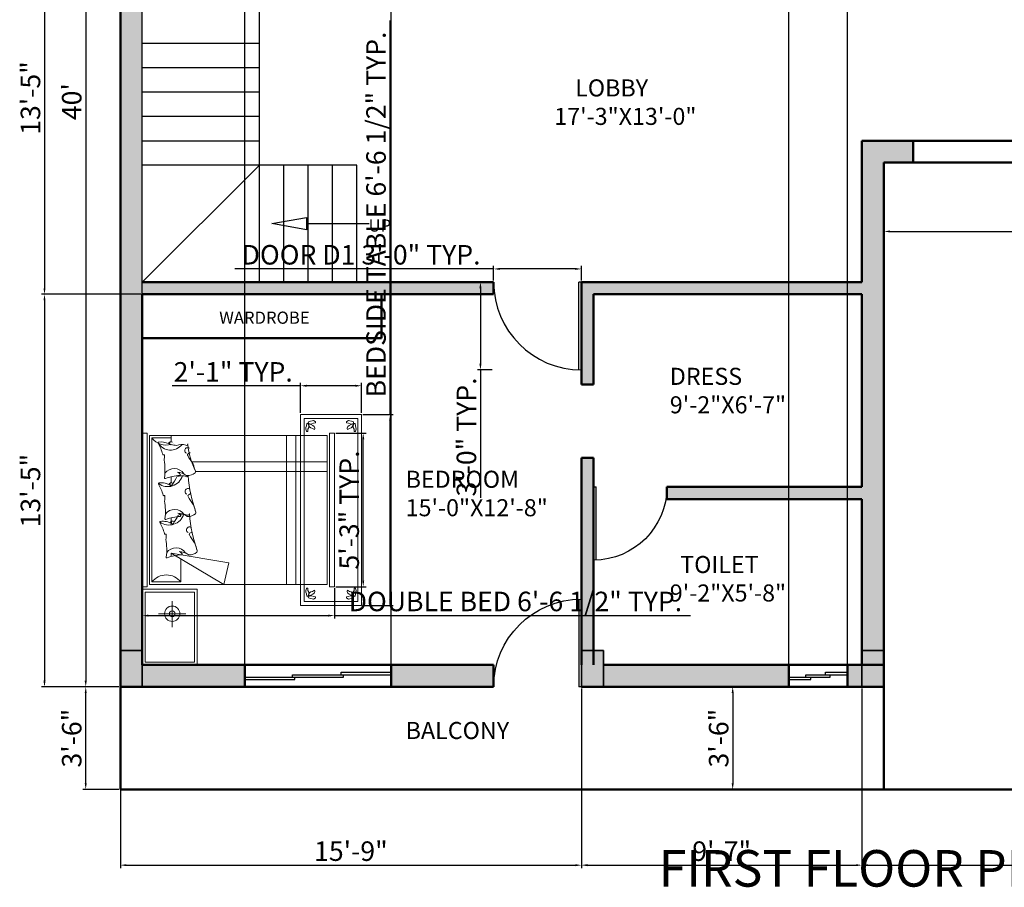
# Model space of a CAD drawing. Units: inches. Extents: x 1770 to 3141, y 984 to 1614.
# Tile 10 of 12: x 2468 to 2871, y 1003 to 1359. Entities that reach past the tile are written whole.
import ezdxf

# ---------------------------------------------------------------- set-up
doc = ezdxf.new("R2010")
doc.units = ezdxf.units.IN
for name, color, linetype, lineweight in [('A-ANNO-DIMS', 2, 'Continuous', 18), ('A-ANNO-TEXT', 7, 'Continuous', 18), ('A-AREA-IDEN', 3, 'Continuous', 18), ('A-COLS', 1, 'Continuous', 35), ('A-DOOR', 4, 'Continuous', 25), ('A-FLOR-STRS', 7, 'Continuous', 25), ('A-FURN', 8, 'Continuous', 18), ('A-GLAZ', 5, 'Continuous', 25), ('A-WALL', 7, 'Continuous', 50), ('A-WALL-PATT', 8, 'Continuous', 13)]:
    doc.layers.add(name, color=color, linetype=linetype, lineweight=lineweight)
doc.styles.get("Standard").update_dxf_attribs({"font": 'arial.ttf'})
doc.dimstyles.new('ISO-25', dxfattribs={"dimtxt": 8, "dimasz": 2.5, "dimexe": 1.25, "dimexo": 0.625, "dimtad": 1, "dimdec": 1, "dimlunit": 3, "dimtxsty": 'Standard', "dimcen": 2.5, "dimclrt": 1, "dimadec": 0, "dimazin": 0, "dimtfac": 1, "dimtdec": 1, "dimtmove": 0, "dimatfit": 3, "dimfxl": 1, "dimarcsym": 0})

# ---------------------------------------------------------------- blocks, each defined once
blk = doc.blocks.new('*D19')
at = {"layer": 'A-ANNO-DIMS', "color": 0, "lineweight": -2, "transparency": 16777216}
for p, q in [((2508.45, 1565.18), (2493.64, 1565.18)), ((2494.89, 1562.68), (2494.89, 1087.68)), ((2508.45, 1085.18), (2493.64, 1085.18))]:
    blk.add_line(p, q, dxfattribs=at)
at = {"layer": 'A-ANNO-DIMS', "color": 0, "transparency": 16777216}
for points in [[(2494.47, 1562.68), (2495.3, 1562.68), (2494.89, 1565.18)], [(2494.47, 1087.68), (2495.3, 1087.68), (2494.89, 1085.18)]]:
    blk.add_solid(points, dxfattribs=at)
at = {"layer": 'Defpoints', "color": 0, "transparency": 16777216}
for p in [(2509.08, 1565.18), (2494.89, 1085.18), (2509.08, 1085.18)]:
    blk.add_point(p, dxfattribs=at)
at = {"layer": 'A-ANNO-DIMS', "color": 0, "transparency": 16777216, "insert": (2490.18, 1325.18), "char_height": 8, "attachment_point": 5, "rotation": 90}
blk.add_mtext("40'", dxfattribs=at)
blk = doc.blocks.new('*D22')
at = {"layer": 'A-ANNO-DIMS', "color": 0, "lineweight": -2, "transparency": 16777216}
for p, q in [((2508.45, 1085.18), (2493.64, 1085.18)), ((2494.89, 1045.68), (2494.89, 1082.68)), ((2508.45, 1043.18), (2493.64, 1043.18))]:
    blk.add_line(p, q, dxfattribs=at)
at = {"layer": 'A-ANNO-DIMS', "color": 0, "transparency": 16777216}
for points in [[(2494.47, 1082.68), (2495.3, 1082.68), (2494.89, 1085.18)], [(2494.47, 1045.68), (2495.3, 1045.68), (2494.89, 1043.18)]]:
    blk.add_solid(points, dxfattribs=at)
at = {"layer": 'Defpoints', "color": 0, "transparency": 16777216}
for p in [(2494.89, 1085.18), (2509.08, 1085.18), (2509.08, 1043.18)]:
    blk.add_point(p, dxfattribs=at)
at = {"layer": 'A-ANNO-DIMS', "color": 0, "transparency": 16777216, "insert": (2490.17, 1064.18), "char_height": 8, "attachment_point": 5, "rotation": 90}
blk.add_mtext('3\'-6"', dxfattribs=at)
blk = doc.blocks.new("D1 3'")
for p, q in [((0, 36), (0, 0)), ((1, 36), (1, 0)), ((0, 0), (1, 0))]:
    blk.add_line(p, q)
blk.add_arc((0, 0), 36, 0, 90)
blk = doc.blocks.new("D2 2'6")
for p, q in [((0, 30), (0, 0)), ((1, 30), (1, 0)), ((0, 0), (1, 0))]:
    blk.add_line(p, q)
blk.add_arc((0, 0), 30, 0, 90)
blk = doc.blocks.new('carpet-7')
at = {"color": 0, "linetype": 'ByBlock'}
for p, q in [((-1.0224, 0), (0, 0)), ((0, 0), (0, -0.54)), ((-1.694, -0.54), (-1.694, 0)), ((-1.694, 0), (-1.0224, 0)), ((-1.658, -0.5076), (-1.658, -0.0324)), ((-1.658, -0.0324), (-0.036, -0.0324)), ((-1.6304, -0.0896), (-1.6256, -0.0702)), ((-1.6256, -0.0702), (-1.6172, -0.0691)), ((-1.6172, -0.0691), (-1.6124, -0.0724)), ((-1.6112, -0.0562), (-1.6124, -0.0637)), ((-1.6124, -0.0637), (-1.6088, -0.068)), ((-1.6124, -0.0724), (-1.6064, -0.0886)), ((-1.5896, -0.0518), (-1.6112, -0.0562)), ((-1.6088, -0.068), (-1.5908, -0.0734)), ((-1.6088, -0.0788), (-1.6028, -0.0724)), ((-1.5992, -0.0961), (-1.6088, -0.0788)), ((-1.6028, -0.0724), (-1.5968, -0.0724)), ((-1.5968, -0.0724), (-1.5812, -0.081)), ((-1.5908, -0.0734), (-1.5764, -0.0724)), ((-1.5752, -0.0486), (-1.5896, -0.0518)), ((-1.5812, -0.081), (-1.5728, -0.0918)), ((-1.5764, -0.0724), (-1.5608, -0.0659)), ((-1.5608, -0.0464), (-1.5752, -0.0486)), ((-1.544, -0.0529), (-1.5608, -0.0464)), ((-1.5608, -0.0659), (-1.5404, -0.0637)), ((-1.5404, -0.0562), (-1.544, -0.0529)), ((-1.5404, -0.0637), (-1.5404, -0.0562)), ((-0.1512, -0.0562), (-0.1476, -0.0529)), ((-0.1512, -0.0637), (-0.1512, -0.0562)), ((-0.1308, -0.0659), (-0.1512, -0.0637)), ((-0.1476, -0.0529), (-0.1308, -0.0464)), ((-0.1308, -0.0464), (-0.1164, -0.0486)), ((-0.1152, -0.0724), (-0.1308, -0.0659)), ((-0.1104, -0.081), (-0.1188, -0.0918)), ((-0.1164, -0.0486), (-0.102, -0.0518)), ((-0.1008, -0.0734), (-0.1152, -0.0724)), ((-0.0948, -0.0724), (-0.1104, -0.081)), ((-0.102, -0.0518), (-0.0804, -0.0562)), ((-0.0828, -0.068), (-0.1008, -0.0734)), ((-0.0888, -0.0724), (-0.0948, -0.0724)), ((-0.0924, -0.0961), (-0.0828, -0.0788)), ((-0.0828, -0.0788), (-0.0888, -0.0724)), ((-0.0792, -0.0724), (-0.0852, -0.0886)), ((-0.0792, -0.0637), (-0.0828, -0.068)), ((-0.0804, -0.0562), (-0.0792, -0.0637)), ((-0.0744, -0.0691), (-0.0792, -0.0724)), ((-0.066, -0.0702), (-0.0744, -0.0691)), ((-0.0612, -0.0896), (-0.066, -0.0702)), ((-0.036, -0.0324), (-0.036, -0.5076)), ((-1.6364, -0.1156), (-1.634, -0.1026)), ((-1.6292, -0.1307), (-1.6364, -0.1156)), ((-1.634, -0.1026), (-1.6304, -0.0896)), ((-1.6256, -0.1339), (-1.6292, -0.1307)), ((-1.6172, -0.1339), (-1.6256, -0.1339)), ((-1.6148, -0.1156), (-1.6172, -0.1339)), ((-1.6076, -0.1015), (-1.6148, -0.1156)), ((-1.6064, -0.0886), (-1.6076, -0.1015)), ((-1.5932, -0.108), (-1.5992, -0.0961)), ((-1.5848, -0.1199), (-1.5932, -0.108)), ((-1.5692, -0.1274), (-1.5848, -0.1199)), ((-1.5728, -0.0918), (-1.568, -0.1069)), ((-1.5632, -0.1274), (-1.5692, -0.1274)), ((-1.568, -0.1069), (-1.5572, -0.1231)), ((-1.5572, -0.1231), (-1.5632, -0.1274)), ((-0.1236, -0.1069), (-0.1344, -0.1231)), ((-0.1344, -0.1231), (-0.1284, -0.1274)), ((-0.1284, -0.1274), (-0.1224, -0.1274)), ((-0.1188, -0.0918), (-0.1236, -0.1069)), ((-0.1224, -0.1274), (-0.1068, -0.1199)), ((-0.1068, -0.1199), (-0.0984, -0.108)), ((-0.0984, -0.108), (-0.0924, -0.0961)), ((-0.0852, -0.0886), (-0.084, -0.1015)), ((-0.084, -0.1015), (-0.0768, -0.1156)), ((-0.0768, -0.1156), (-0.0744, -0.1339)), ((-0.0744, -0.1339), (-0.066, -0.1339)), ((-0.066, -0.1339), (-0.0624, -0.1307)), ((-0.0624, -0.1307), (-0.0552, -0.1156)), ((-0.0576, -0.1026), (-0.0612, -0.0896)), ((-0.0552, -0.1156), (-0.0576, -0.1026)), ((-1.6292, -0.4093), (-1.6364, -0.4244)), ((-1.6364, -0.4244), (-1.634, -0.4374)), ((-1.6256, -0.4061), (-1.6292, -0.4093)), ((-1.6172, -0.4061), (-1.6256, -0.4061)), ((-1.6148, -0.4244), (-1.6172, -0.4061)), ((-1.6076, -0.4385), (-1.6148, -0.4244)), ((-1.5932, -0.432), (-1.5992, -0.4439)), ((-1.5848, -0.4201), (-1.5932, -0.432)), ((-1.5692, -0.4126), (-1.5848, -0.4201)), ((-1.5728, -0.4482), (-1.568, -0.4331)), ((-1.5632, -0.4126), (-1.5692, -0.4126)), ((-1.568, -0.4331), (-1.5572, -0.4169)), ((-1.5572, -0.4169), (-1.5632, -0.4126)), ((-0.1344, -0.4169), (-0.1284, -0.4126)), ((-0.1236, -0.4331), (-0.1344, -0.4169)), ((-0.1284, -0.4126), (-0.1224, -0.4126)), ((-0.1188, -0.4482), (-0.1236, -0.4331)), ((-0.1224, -0.4126), (-0.1068, -0.4201)), ((-0.1068, -0.4201), (-0.0984, -0.432)), ((-0.0984, -0.432), (-0.0924, -0.4439)), ((-0.084, -0.4385), (-0.0768, -0.4244)), ((-0.0768, -0.4244), (-0.0744, -0.4061)), ((-0.0744, -0.4061), (-0.066, -0.4061)), ((-0.066, -0.4061), (-0.0624, -0.4093)), ((-0.0624, -0.4093), (-0.0552, -0.4244)), ((-0.0552, -0.4244), (-0.0576, -0.4374)), ((-1.658, -0.5076), (-0.036, -0.5076)), ((-1.634, -0.4374), (-1.6304, -0.4504)), ((-1.6304, -0.4504), (-1.6256, -0.4698)), ((-1.6256, -0.4698), (-1.6172, -0.4709)), ((-1.6172, -0.4709), (-1.6124, -0.4676)), ((-1.6124, -0.4676), (-1.6064, -0.4514)), ((-1.6124, -0.4763), (-1.6088, -0.472)), ((-1.6112, -0.4838), (-1.6124, -0.4763)), ((-1.5896, -0.4882), (-1.6112, -0.4838)), ((-1.5992, -0.4439), (-1.6088, -0.4612)), ((-1.6088, -0.4612), (-1.6028, -0.4676)), ((-1.6088, -0.472), (-1.5908, -0.4666)), ((-1.6064, -0.4514), (-1.6076, -0.4385)), ((-1.6028, -0.4676), (-1.5968, -0.4676)), ((-1.5968, -0.4676), (-1.5812, -0.459)), ((-1.5908, -0.4666), (-1.5764, -0.4676)), ((-1.5752, -0.4914), (-1.5896, -0.4882)), ((-1.5812, -0.459), (-1.5728, -0.4482)), ((-1.5764, -0.4676), (-1.5608, -0.4741)), ((-1.5608, -0.4936), (-1.5752, -0.4914)), ((-1.5608, -0.4741), (-1.5404, -0.4763)), ((-1.544, -0.4871), (-1.5608, -0.4936)), ((-1.5404, -0.4838), (-1.544, -0.4871)), ((-1.5404, -0.4763), (-1.5404, -0.4838)), ((-0.1308, -0.4741), (-0.1512, -0.4763)), ((-0.1512, -0.4763), (-0.1512, -0.4838)), ((-0.1512, -0.4838), (-0.1476, -0.4871)), ((-0.1476, -0.4871), (-0.1308, -0.4936)), ((-0.1152, -0.4676), (-0.1308, -0.4741)), ((-0.1308, -0.4936), (-0.1164, -0.4914)), ((-0.1104, -0.459), (-0.1188, -0.4482)), ((-0.1164, -0.4914), (-0.102, -0.4882)), ((-0.1008, -0.4666), (-0.1152, -0.4676)), ((-0.0948, -0.4676), (-0.1104, -0.459)), ((-0.102, -0.4882), (-0.0804, -0.4838)), ((-0.0828, -0.472), (-0.1008, -0.4666)), ((-0.0888, -0.4676), (-0.0948, -0.4676)), ((-0.0924, -0.4439), (-0.0828, -0.4612)), ((-0.0828, -0.4612), (-0.0888, -0.4676)), ((-0.0852, -0.4514), (-0.084, -0.4385)), ((-0.0792, -0.4676), (-0.0852, -0.4514)), ((-0.0792, -0.4763), (-0.0828, -0.472)), ((-0.0804, -0.4838), (-0.0792, -0.4763)), ((-0.0744, -0.4709), (-0.0792, -0.4676)), ((-0.066, -0.4698), (-0.0744, -0.4709)), ((-0.0612, -0.4504), (-0.066, -0.4698)), ((-0.0576, -0.4374), (-0.0612, -0.4504)), ((0, -0.54), (-1.694, -0.54))]:
    blk.add_line(p, q, dxfattribs=at)
blk = doc.blocks.new('*D51')
at = {"layer": 'A-ANNO-DIMS', "color": 0, "lineweight": -2, "transparency": 16777216}
for p, q in [((2760.08, 1082.68), (2760.08, 1045.68)), ((2760.7, 1085.18), (2761.33, 1085.18)), ((2760.7, 1043.18), (2761.33, 1043.18))]:
    blk.add_line(p, q, dxfattribs=at)
at = {"layer": 'A-ANNO-DIMS', "color": 0, "transparency": 16777216}
for points in [[(2759.66, 1082.68), (2760.5, 1082.68), (2760.08, 1085.18)], [(2759.66, 1045.68), (2760.5, 1045.68), (2760.08, 1043.18)]]:
    blk.add_solid(points, dxfattribs=at)
at = {"layer": 'Defpoints', "color": 0, "transparency": 16777216}
for p in [(2760.08, 1085.18), (2760.08, 1043.18), (2760.08, 1043.18)]:
    blk.add_point(p, dxfattribs=at)
at = {"layer": 'A-ANNO-DIMS', "color": 0, "transparency": 16777216, "insert": (2755.37, 1064.18), "char_height": 8, "attachment_point": 5, "rotation": 90}
blk.add_mtext('3\'-6"', dxfattribs=at)
blk = doc.blocks.new('*D52')
at = {"layer": 'A-ANNO-DIMS', "color": 0, "lineweight": -2, "transparency": 16777216}
for p, q in [((2822.08, 1274.4), (2822.08, 1270.71)), ((2824.58, 1271.96), (3097.58, 1271.96)), ((3100.08, 1274.4), (3100.08, 1270.71))]:
    blk.add_line(p, q, dxfattribs=at)
at = {"layer": 'A-ANNO-DIMS', "color": 0, "transparency": 16777216}
for points in [[(2824.58, 1272.38), (2824.58, 1271.54), (2822.08, 1271.96)], [(3097.58, 1272.38), (3097.58, 1271.54), (3100.08, 1271.96)]]:
    blk.add_solid(points, dxfattribs=at)
at = {"layer": 'Defpoints', "color": 0, "transparency": 16777216}
for p in [(2822.08, 1275.03), (3100.08, 1275.03), (3100.08, 1271.96)]:
    blk.add_point(p, dxfattribs=at)
at = {"layer": 'A-ANNO-DIMS', "color": 0, "transparency": 16777216, "insert": (2961.08, 1276.67), "char_height": 8, "attachment_point": 5}
blk.add_mtext('23\'-2"', dxfattribs=at)
blk = doc.blocks.new('BED-DOUBLE')
for p, q in [((3.94, 1.97), (3.94, 61.02)), ((3.94, 61.02), (11.81, 61.02)), ((11.81, 62.01), (11.81, 59.48)), ((59.06, 0.98), (59.06, 62.01)), ((62.99, 0.98), (62.99, 62.01)), ((20.58, 51.18), (75.79, 51.18)), ((11.81, 45.13), (11.81, 42.7)), ((21.83, 47.24), (75.79, 47.24)), ((11.81, 28.3), (11.81, 26.75)), ((11.81, 13.78), (33.46, 0.98)), ((35.43, 9.84), (11.81, 13.78)), ((11.81, 12.41), (11.81, 13.78)), ((15.75, 1.97), (15.75, 11.45)), ((33.46, 0.98), (35.43, 9.84)), ((3.94, 1.97), (15.75, 1.97))]:
    blk.add_line(p, q)
for points in [[(1.97, 0), (1.97, 62.99), (0, 62.99), (0, 0)], [(75.79, 62.01), (2.95, 62.01), (2.95, 0.98), (75.79, 0.98)], [(78.74, 0), (78.74, 62.99), (76.77, 62.99), (76.77, 0)]]:
    blk.add_lwpolyline(points, close=True)
for centre, radius, start, end in [((9.84, 65.6), 7.47, 217.7826, 285.2747), ((6.72, 59.06), 0.283, 97.124, 208.2114), ((6.72, 59.06), 0.283, 97.124, 208.2114), ((11.6, 61.98), 5.92, 209.3598, 322.4281), ((-14.44, 47.71), 23.73, 16.2196, 28.2114), ((7.62, 51.84), 7.55, 66.1093, 97.124), ((11.74, 58.34), 1.13, 52.662, 159.1573), ((74.55, 55.49), 63.42, 176.4982, 177.2888), ((11.63, 58.56), 0.283, 218.8315, 325.8329), ((16.48, 74.25), 16.51, 253.7524, 261.4605), ((-45.71, 34.29), 63.42, 22.7018, 22.7206), ((16.03, 53.78), 4.59, 67.1663, 115.7613), ((18.58, 55.86), 1.2, 52.3565, 245.7762), ((18.03, 58.54), 0.567, 247.1663, 4.3422), ((51.64, 61.93), 33.22, 186.224, 206.0326), ((8.62, 54.41), 0.283, 196.2196, 290.689), ((8.82, 53.88), 0.283, 359.3085, 110.689), ((-2.22, 54.02), 11.32, 349.4168, 359.3085), ((19.09, 54.05), 0.567, 102.6426, 209.049), ((41.54, 66.52), 26.25, 209.049, 217.3823), ((18.84, 55.16), 0.567, 282.6426, 292.7015), ((18.58, 55.79), 1.26, 292.7015, 327.1556), ((-14.44, 47.71), 23.73, 352.7248, 10.2702), ((13.07, 43.78), 4.71, 32.7628, 143.8922), ((20.28, 50.19), 0.567, 16.386, 43.7955), ((77.39, 66.98), 58.96, 196.386, 199.4465), ((10.39, 47.46), 6.39, 233.8947, 342.3952), ((9.38, 44.67), 0.283, 172.7248, 290.959), ((16.23, 26.77), 18.88, 92.7363, 110.959), ((-34.15, 72.98), 55.83, 325.8329, 330.0245), ((16.21, 40.94), 4.59, 67.1663, 115.7613), ((14.36, 41.08), 5.89, 51.6071, 89.7845), ((13.92, 45.16), 1.87, 28.2985, 75.7891), ((15.32, 45.91), 0.283, 272.7363, 28.2985), ((18.22, 45.7), 0.567, 247.1663, 4.3422), ((18.37, 46.14), 0.567, 231.6071, 267.3377), ((18.56, 50.2), 4.62, 267.3377, 311.666), ((77.57, 50.21), 58.96, 184.5852, 199.4465), ((21.25, 47.17), 0.567, 311.666, 19.4465), ((6.91, 42.28), 0.283, 97.124, 208.2114), ((6.91, 42.28), 0.283, 97.124, 208.2114), ((-14.25, 30.93), 23.73, 16.2196, 28.2114), ((7.81, 35.07), 7.55, 59.9211, 97.124), ((11.93, 41.57), 1.13, 52.662, 159.1573), ((74.73, 38.72), 63.42, 176.4982, 177.2888), ((11.81, 41.78), 0.283, 218.8315, 325.8329), ((-45.53, 17.51), 63.42, 22.7018, 22.7206), ((8.8, 37.64), 0.283, 196.2196, 290.689), ((9, 37.11), 0.283, 359.3085, 110.689), ((-2.03, 37.24), 11.32, 349.4168, 359.3085), ((18.76, 39.09), 1.2, 52.3565, 245.7762), ((19.28, 37.27), 0.567, 102.6426, 209.049), ((41.73, 49.74), 26.25, 209.049, 217.3823), ((19.03, 38.38), 0.567, 282.6426, 292.7015), ((18.76, 39.02), 1.26, 292.7015, 327.1556), ((-14.25, 30.93), 23.73, 352.7248, 10.2702), ((20.46, 33.41), 0.567, 16.386, 43.7955), ((77.57, 50.21), 58.96, 196.386, 199.4465), ((10.93, 31.72), 6.39, 233.8947, 342.3952), ((13.25, 27), 4.71, 32.7628, 143.8922), ((16.42, 9.99), 18.88, 92.7363, 110.959), ((-33.61, 57.23), 55.83, 325.8329, 330.0245), ((14.54, 24.31), 5.89, 51.6071, 89.7845), ((14.11, 28.38), 1.87, 28.2985, 75.7891), ((16.75, 25.2), 4.59, 67.1663, 115.7613), ((15.5, 29.14), 0.283, 272.7363, 28.2985), ((18.56, 29.37), 0.567, 231.6071, 267.3377), ((18.75, 29.96), 0.567, 247.1663, 4.3422), ((18.74, 33.42), 4.62, 267.3377, 311.666), ((78.11, 34.46), 58.96, 184.5852, 199.4465), ((21.44, 30.39), 0.567, 311.666, 19.4465), ((7.44, 26.53), 0.283, 97.124, 208.2114), ((7.44, 26.53), 0.283, 97.124, 208.2114), ((-13.71, 15.19), 23.73, 16.2196, 28.2114), ((8.35, 19.32), 7.55, 59.9211, 97.124), ((9.56, 27.89), 0.283, 172.7248, 290.959), ((12.47, 25.82), 1.13, 52.662, 159.1573), ((75.27, 22.97), 63.42, 176.4982, 177.2888), ((12.35, 26.04), 0.283, 218.8315, 325.8329), ((-44.99, 1.77), 63.42, 22.7018, 22.7206), ((19.3, 23.34), 1.2, 52.3565, 245.7762), ((9.34, 21.89), 0.283, 196.2196, 290.689), ((9.54, 21.36), 0.283, 359.3085, 110.689), ((-1.49, 21.49), 11.32, 349.4168, 359.3085), ((19.82, 21.53), 0.567, 102.6426, 209.049), ((42.27, 34), 26.25, 209.049, 217.3823), ((19.57, 22.63), 0.567, 282.6426, 292.7015), ((19.3, 23.27), 1.26, 292.7015, 327.1556), ((-13.71, 15.19), 23.73, 352.7248, 10.2702), ((21, 17.67), 0.567, 16.386, 43.7955), ((78.11, 34.46), 58.96, 196.386, 199.4465), ((10.1, 12.14), 0.283, 172.7248, 290.959), ((13.79, 11.26), 4.71, 32.7628, 143.8922), ((16.96, -5.75), 18.88, 92.7363, 110.959), ((15.08, 8.56), 5.89, 51.6071, 89.7845), ((14.65, 12.64), 1.87, 28.2985, 75.7891), ((16.04, 13.39), 0.283, 272.7363, 28.2985), ((19.09, 13.62), 0.567, 231.6071, 267.3377), ((19.28, 17.67), 4.62, 267.3377, 311.666), ((21.98, 14.64), 0.567, 311.666, 19.4465), ((9.84, -2.61), 7.47, 37.7826, 142.2174)]:
    blk.add_arc(centre, radius, start, end)
blk = doc.blocks.new('COLUMN-9x15')
at = {"transparency": 33554687}
h = blk.add_hatch(color=256, dxfattribs=at)
h.dxf.hatch_style = 1
h.paths.add_polyline_path([(9, 15), (0, 15), (0, 0), (9, 0)])
blk.add_lwpolyline([(9, 15), (0, 15), (0, 0), (9, 0)], close=True)
blk = doc.blocks.new('*D72')
at = {"layer": 'A-ANNO-DIMS', "color": 0, "lineweight": -2, "transparency": 16777216}
for p, q in [((2662.08, 1256.58), (2555.94, 1256.58)), ((2662.08, 1251.8), (2662.08, 1257.83)), ((2695.58, 1256.58), (2664.58, 1256.58)), ((2698.08, 1251.8), (2698.08, 1257.83))]:
    blk.add_line(p, q, dxfattribs=at)
at = {"layer": 'A-ANNO-DIMS', "color": 0, "transparency": 16777216}
for points in [[(2664.58, 1257), (2664.58, 1256.16), (2662.08, 1256.58)], [(2695.58, 1257), (2695.58, 1256.16), (2698.08, 1256.58)]]:
    blk.add_solid(points, dxfattribs=at)
at = {"layer": 'Defpoints', "color": 0, "transparency": 16777216}
for p in [(2662.08, 1256.58), (2662.08, 1251.18), (2698.08, 1251.18)]:
    blk.add_point(p, dxfattribs=at)
at = {"layer": 'A-ANNO-DIMS', "color": 1, "transparency": 16777216, "insert": (2607.76, 1261.35), "char_height": 8, "attachment_point": 5}
blk.add_mtext('DOOR D1 3\'-0" TYP.', dxfattribs=at)
blk = doc.blocks.new('*D73')
at = {"layer": 'A-ANNO-DIMS', "color": 0, "lineweight": -2, "transparency": 16777216}
for p, q in [((2661.45, 1251.18), (2655.43, 1251.18)), ((2656.68, 1248.68), (2656.68, 1217.68)), ((2661.45, 1215.18), (2655.43, 1215.18)), ((2656.68, 1215.18), (2656.68, 1162.67))]:
    blk.add_line(p, q, dxfattribs=at)
at = {"layer": 'A-ANNO-DIMS', "color": 0, "transparency": 16777216}
for points in [[(2656.26, 1248.68), (2657.1, 1248.68), (2656.68, 1251.18)], [(2656.26, 1217.68), (2657.1, 1217.68), (2656.68, 1215.18)]]:
    blk.add_solid(points, dxfattribs=at)
at = {"layer": 'Defpoints', "color": 0, "transparency": 16777216}
for p in [(2662.08, 1251.18), (2656.68, 1215.18), (2662.08, 1215.18)]:
    blk.add_point(p, dxfattribs=at)
at = {"layer": 'A-ANNO-DIMS', "color": 1, "transparency": 16777216, "insert": (2651.97, 1187.67), "char_height": 8, "attachment_point": 5, "rotation": 90}
blk.add_mtext('3\'-0" TYP.', dxfattribs=at)
blk = doc.blocks.new('*D78')
at = {"layer": 'A-ANNO-DIMS', "color": 0, "lineweight": -2, "transparency": 16777216}
for p, q in [((2619.67, 1196.93), (2619.67, 1358.41)), ((2608.53, 1196.93), (2620.92, 1196.93)), ((2619.67, 1121.04), (2619.67, 1194.43)), ((2608.53, 1118.54), (2620.92, 1118.54))]:
    blk.add_line(p, q, dxfattribs=at)
at = {"layer": 'A-ANNO-DIMS', "color": 0, "transparency": 16777216}
for points in [[(2619.25, 1194.43), (2620.08, 1194.43), (2619.67, 1196.93)], [(2619.25, 1121.04), (2620.08, 1121.04), (2619.67, 1118.54)]]:
    blk.add_solid(points, dxfattribs=at)
at = {"layer": 'Defpoints', "color": 0, "transparency": 16777216}
for p in [(2607.91, 1196.93), (2619.67, 1196.93), (2607.91, 1118.54)]:
    blk.add_point(p, dxfattribs=at)
at = {"layer": 'A-ANNO-DIMS', "color": 1, "transparency": 16777216, "insert": (2614.91, 1278.92), "char_height": 8, "attachment_point": 5, "rotation": 90}
blk.add_mtext('BEDSIDE TABLE 6\'-6 1/2" TYP.', dxfattribs=at)
blk = doc.blocks.new('*D79')
at = {"layer": 'A-ANNO-DIMS', "color": 0, "lineweight": -2, "transparency": 16777216}
for p, q in [((2582.92, 1208.69), (2530.27, 1208.69)), ((2582.92, 1197.55), (2582.92, 1209.94)), ((2605.41, 1208.69), (2585.42, 1208.69)), ((2607.91, 1197.55), (2607.91, 1209.94))]:
    blk.add_line(p, q, dxfattribs=at)
at = {"layer": 'A-ANNO-DIMS', "color": 0, "transparency": 16777216}
for points in [[(2585.42, 1209.1), (2585.42, 1208.27), (2582.92, 1208.69)], [(2605.41, 1209.1), (2605.41, 1208.27), (2607.91, 1208.69)]]:
    blk.add_solid(points, dxfattribs=at)
at = {"layer": 'Defpoints', "color": 0, "transparency": 16777216}
for p in [(2582.92, 1208.69), (2582.92, 1196.93), (2607.91, 1196.93)]:
    blk.add_point(p, dxfattribs=at)
at = {"layer": 'A-ANNO-DIMS', "color": 1, "transparency": 16777216, "insert": (2555.34, 1213.33), "char_height": 8, "attachment_point": 5}
blk.add_mtext('2\'-1" TYP.', dxfattribs=at)
blk = doc.blocks.new('*D80')
at = {"layer": 'A-ANNO-DIMS', "color": 0, "lineweight": -2, "transparency": 16777216}
for p, q in [((2518.08, 1125.61), (2518.08, 1113.18)), ((2596.82, 1125.61), (2596.82, 1113.18)), ((2520.58, 1114.43), (2594.32, 1114.43)), ((2596.82, 1114.43), (2742.72, 1114.43))]:
    blk.add_line(p, q, dxfattribs=at)
at = {"layer": 'A-ANNO-DIMS', "color": 0, "transparency": 16777216}
for points in [[(2520.58, 1114.84), (2520.58, 1114.01), (2518.08, 1114.43)], [(2594.32, 1114.84), (2594.32, 1114.01), (2596.82, 1114.43)]]:
    blk.add_solid(points, dxfattribs=at)
at = {"layer": 'Defpoints', "color": 0, "transparency": 16777216}
for p in [(2518.08, 1126.24), (2596.82, 1126.24), (2596.82, 1114.43)]:
    blk.add_point(p, dxfattribs=at)
at = {"layer": 'A-ANNO-DIMS', "color": 1, "transparency": 16777216, "insert": (2671.02, 1119.19), "char_height": 8, "attachment_point": 5}
blk.add_mtext('DOUBLE BED 6\'-6 1/2" TYP.', dxfattribs=at)
blk = doc.blocks.new('*D81')
at = {"layer": 'A-ANNO-DIMS', "color": 0, "lineweight": -2, "transparency": 16777216}
for p, q in [((2597.44, 1189.23), (2609.88, 1189.23)), ((2608.63, 1128.74), (2608.63, 1186.73)), ((2597.44, 1126.24), (2609.88, 1126.24))]:
    blk.add_line(p, q, dxfattribs=at)
at = {"layer": 'A-ANNO-DIMS', "color": 0, "transparency": 16777216}
for points in [[(2608.21, 1186.73), (2609.05, 1186.73), (2608.63, 1189.23)], [(2608.21, 1128.74), (2609.05, 1128.74), (2608.63, 1126.24)]]:
    blk.add_solid(points, dxfattribs=at)
at = {"layer": 'Defpoints', "color": 0, "transparency": 16777216}
for p in [(2596.82, 1189.23), (2608.63, 1189.23), (2596.82, 1126.24)]:
    blk.add_point(p, dxfattribs=at)
at = {"layer": 'A-ANNO-DIMS', "color": 1, "transparency": 16777216, "insert": (2603.92, 1157.74), "char_height": 8, "attachment_point": 5, "rotation": 90}
blk.add_mtext('5\'-3" TYP.', dxfattribs=at)
blk = doc.blocks.new('*D129')
at = {"layer": 'A-ANNO-DIMS', "color": 0, "lineweight": -2, "transparency": 16777216}
for p, q in [((2517.45, 1407.18), (2476.73, 1407.18)), ((2477.98, 1404.68), (2477.98, 1248.68)), ((2517.45, 1246.18), (2476.73, 1246.18))]:
    blk.add_line(p, q, dxfattribs=at)
at = {"layer": 'A-ANNO-DIMS', "color": 0, "transparency": 16777216}
for points in [[(2477.56, 1404.68), (2478.4, 1404.68), (2477.98, 1407.18)], [(2477.56, 1248.68), (2478.4, 1248.68), (2477.98, 1246.18)]]:
    blk.add_solid(points, dxfattribs=at)
at = {"layer": 'Defpoints', "color": 0, "transparency": 16777216}
for p in [(2518.08, 1407.18), (2477.98, 1246.18), (2518.08, 1246.18)]:
    blk.add_point(p, dxfattribs=at)
at = {"layer": 'A-ANNO-DIMS', "color": 1, "transparency": 16777216, "insert": (2473.27, 1326.68), "char_height": 8, "attachment_point": 5, "rotation": 90}
blk.add_mtext('13\'-5"', dxfattribs=at)
blk = doc.blocks.new('*D130')
at = {"layer": 'A-ANNO-DIMS', "color": 0, "lineweight": -2, "transparency": 16777216}
for p, q in [((2517.45, 1246.18), (2476.73, 1246.18)), ((2477.98, 1243.68), (2477.98, 1087.68)), ((2508.45, 1085.18), (2476.73, 1085.18))]:
    blk.add_line(p, q, dxfattribs=at)
at = {"layer": 'A-ANNO-DIMS', "color": 0, "transparency": 16777216}
for points in [[(2477.56, 1243.68), (2478.4, 1243.68), (2477.98, 1246.18)], [(2477.56, 1087.68), (2478.4, 1087.68), (2477.98, 1085.18)]]:
    blk.add_solid(points, dxfattribs=at)
at = {"layer": 'Defpoints', "color": 0, "transparency": 16777216}
for p in [(2518.08, 1246.18), (2477.98, 1085.18), (2509.08, 1085.18)]:
    blk.add_point(p, dxfattribs=at)
at = {"layer": 'A-ANNO-DIMS', "color": 1, "transparency": 16777216, "insert": (2473.27, 1165.68), "char_height": 8, "attachment_point": 5, "rotation": 90}
blk.add_mtext('13\'-5"', dxfattribs=at)
blk = doc.blocks.new('*D131')
at = {"layer": 'A-ANNO-DIMS', "color": 0, "lineweight": -2, "transparency": 16777216}
for p, q in [((2509.08, 1084.55), (2509.08, 1010.83)), ((2698.08, 1084.55), (2698.08, 1010.83)), ((2511.58, 1012.08), (2695.58, 1012.08))]:
    blk.add_line(p, q, dxfattribs=at)
at = {"layer": 'A-ANNO-DIMS', "color": 0, "transparency": 16777216}
for points in [[(2511.58, 1012.5), (2511.58, 1011.66), (2509.08, 1012.08)], [(2695.58, 1012.5), (2695.58, 1011.66), (2698.08, 1012.08)]]:
    blk.add_solid(points, dxfattribs=at)
at = {"layer": 'Defpoints', "color": 0, "transparency": 16777216}
for p in [(2509.08, 1085.18), (2698.08, 1085.18), (2698.08, 1012.08)]:
    blk.add_point(p, dxfattribs=at)
at = {"layer": 'A-ANNO-DIMS', "color": 1, "transparency": 16777216, "insert": (2603.58, 1016.79), "char_height": 8, "attachment_point": 5}
blk.add_mtext('15\'-9"', dxfattribs=at)
blk = doc.blocks.new('*D132')
at = {"layer": 'A-ANNO-DIMS', "color": 0, "lineweight": -2, "transparency": 16777216}
for p, q in [((2698.08, 1084.55), (2698.08, 1010.83)), ((2813.08, 1084.55), (2813.08, 1010.83)), ((2700.58, 1012.08), (2810.58, 1012.08))]:
    blk.add_line(p, q, dxfattribs=at)
at = {"layer": 'A-ANNO-DIMS', "color": 0, "transparency": 16777216}
for points in [[(2700.58, 1012.5), (2700.58, 1011.66), (2698.08, 1012.08)], [(2810.58, 1012.5), (2810.58, 1011.66), (2813.08, 1012.08)]]:
    blk.add_solid(points, dxfattribs=at)
at = {"layer": 'Defpoints', "color": 0, "transparency": 16777216}
for p in [(2698.08, 1085.18), (2813.08, 1085.18), (2813.08, 1012.08)]:
    blk.add_point(p, dxfattribs=at)
at = {"layer": 'A-ANNO-DIMS', "color": 1, "transparency": 16777216, "insert": (2755.58, 1016.79), "char_height": 8, "attachment_point": 5}
blk.add_mtext('9\'-7"', dxfattribs=at)
blk = doc.blocks.new('*D133')
at = {"layer": 'A-ANNO-DIMS', "color": 0, "lineweight": -2, "transparency": 16777216}
for p, q in [((2813.08, 1084.55), (2813.08, 1010.83)), ((2977.04, 1084.55), (2977.04, 1010.83)), ((2815.58, 1012.08), (2974.54, 1012.08))]:
    blk.add_line(p, q, dxfattribs=at)
at = {"layer": 'A-ANNO-DIMS', "color": 0, "transparency": 16777216}
for points in [[(2815.58, 1012.5), (2815.58, 1011.66), (2813.08, 1012.08)], [(2974.54, 1012.5), (2974.54, 1011.66), (2977.04, 1012.08)]]:
    blk.add_solid(points, dxfattribs=at)
at = {"layer": 'Defpoints', "color": 0, "transparency": 16777216}
for p in [(2813.08, 1085.18), (2977.04, 1085.18), (2977.04, 1012.08)]:
    blk.add_point(p, dxfattribs=at)
at = {"layer": 'A-ANNO-DIMS', "color": 1, "transparency": 16777216, "insert": (2895.06, 1016.79), "char_height": 8, "attachment_point": 5}
blk.add_mtext('13\'-8"', dxfattribs=at)
blk = doc.blocks.new('*D135')
at = {"layer": 'A-ANNO-DIMS', "color": 0, "lineweight": -2, "transparency": 16777216}
for p, q in [((2518.08, 1094.8), (2518.08, 1597.53)), ((2520.58, 1596.28), (2557.58, 1596.28)), ((2560.08, 1094.8), (2560.08, 1597.53))]:
    blk.add_line(p, q, dxfattribs=at)
at = {"layer": 'A-ANNO-DIMS', "color": 0, "transparency": 16777216}
for points in [[(2520.58, 1596.7), (2520.58, 1595.86), (2518.08, 1596.28)], [(2557.58, 1596.7), (2557.58, 1595.86), (2560.08, 1596.28)]]:
    blk.add_solid(points, dxfattribs=at)
at = {"layer": 'Defpoints', "color": 0, "transparency": 16777216}
for p in [(2560.08, 1596.28), (2518.08, 1094.18), (2560.08, 1094.18)]:
    blk.add_point(p, dxfattribs=at)
at = {"layer": 'A-ANNO-DIMS', "color": 1, "transparency": 16777216, "insert": (2539.08, 1600.99), "char_height": 8, "attachment_point": 5}
blk.add_mtext('3\'-6"', dxfattribs=at)
blk = doc.blocks.new('*D136')
at = {"layer": 'A-ANNO-DIMS', "color": 0, "lineweight": -2, "transparency": 16777216}
for p, q in [((2560.08, 1094.8), (2560.08, 1597.53)), ((2562.58, 1596.28), (2617.58, 1596.28)), ((2620.08, 1094.8), (2620.08, 1597.53))]:
    blk.add_line(p, q, dxfattribs=at)
at = {"layer": 'A-ANNO-DIMS', "color": 0, "transparency": 16777216}
for points in [[(2562.58, 1596.7), (2562.58, 1595.86), (2560.08, 1596.28)], [(2617.58, 1596.7), (2617.58, 1595.86), (2620.08, 1596.28)]]:
    blk.add_solid(points, dxfattribs=at)
at = {"layer": 'Defpoints', "color": 0, "transparency": 16777216}
for p in [(2620.08, 1596.28), (2560.08, 1094.18), (2620.08, 1094.18)]:
    blk.add_point(p, dxfattribs=at)
at = {"layer": 'A-ANNO-DIMS', "color": 1, "transparency": 16777216, "insert": (2590.08, 1600.99), "char_height": 8, "attachment_point": 5}
blk.add_mtext('5\'-0"', dxfattribs=at)
blk = doc.blocks.new('*D137')
at = {"layer": 'A-ANNO-DIMS', "color": 0, "lineweight": -2, "transparency": 16777216}
for p, q in [((2783.08, 1094.8), (2783.08, 1597.53)), ((2785.58, 1596.28), (2804.58, 1596.28)), ((2807.08, 1094.8), (2807.08, 1597.53))]:
    blk.add_line(p, q, dxfattribs=at)
at = {"layer": 'A-ANNO-DIMS', "color": 0, "transparency": 16777216}
for points in [[(2785.58, 1596.7), (2785.58, 1595.86), (2783.08, 1596.28)], [(2804.58, 1596.7), (2804.58, 1595.86), (2807.08, 1596.28)]]:
    blk.add_solid(points, dxfattribs=at)
at = {"layer": 'Defpoints', "color": 0, "transparency": 16777216}
for p in [(2807.08, 1596.28), (2783.08, 1094.18), (2807.08, 1094.18)]:
    blk.add_point(p, dxfattribs=at)
at = {"layer": 'A-ANNO-DIMS', "color": 1, "transparency": 16777216, "insert": (2795.08, 1600.99), "char_height": 8, "attachment_point": 5}
blk.add_mtext('2\'-0"', dxfattribs=at)

msp = doc.modelspace()

# ---------------------------------------------------------------- hatches: boundary and pattern name
at = {"layer": 'A-WALL-PATT'}
h = msp.add_hatch(color=256, dxfattribs=at)
h.dxf.hatch_style = 1
h.paths.add_polyline_path([(2936.08, 1565.18), (2509.08, 1565.18), (2509.08, 1100.18), (2518.08, 1100.18), (2518.08, 1125.25), (2518.08, 1246.18), (2662.08, 1246.18), (2662.08, 1251.18), (2518.08, 1251.18), (2518.08, 1407.18), (2641.08, 1407.18), (2641.08, 1412.18), (2518.08, 1412.18), (2518.08, 1556.18), (2540.6, 1556.18), (2931.08, 1556.18), (2931.08, 1520.18), (2936.08, 1520.18)])
h.paths.add_polyline_path([(2560.08, 1094.18), (2518.08, 1094.18), (2518.08, 1085.18), (2560.08, 1085.18)])
h.paths.add_polyline_path([(2662.08, 1094.18), (2620.08, 1094.18), (2620.08, 1085.18), (2662.08, 1085.18)])
h.paths.add_polyline_path([(2783.08, 1094.18), (2707.08, 1094.18), (2707.08, 1085.18), (2783.08, 1085.18)])
h.paths.add_polyline_path([(2703.08, 1179.18), (2698.08, 1179.18), (2698.08, 1100.18), (2703.08, 1100.18)], flags=16)
h.paths.add_polyline_path([(2813.08, 1094.18), (2807.08, 1094.18), (2807.08, 1085.18), (2813.08, 1085.18)])
h.paths.add_polyline_path([(2822.08, 1300.18), (2834.08, 1300.18), (2834.08, 1309.18), (2813.08, 1309.18), (2813.08, 1251.18), (2698.08, 1251.18), (2698.08, 1215.18), (2698.08, 1209.18), (2703.08, 1209.18), (2703.08, 1246.18), (2813.08, 1246.18), (2813.08, 1167.18), (2733.08, 1167.18), (2733.08, 1162.18), (2813.08, 1162.18), (2813.08, 1100.18), (2822.08, 1100.18)], flags=17)
h.paths.add_polyline_path([(2936.08, 1376.18), (2931.08, 1376.18), (2931.08, 1309.18), (2918.08, 1309.18), (2918.08, 1300.18), (2936.08, 1300.18)], flags=17)
h.paths.add_polyline_path([(2735.08, 1520.18), (2718.08, 1520.18), (2718.08, 1515.18), (2730.08, 1515.18), (2730.08, 1412.18), (2682.08, 1412.18), (2682.08, 1448.18), (2677.08, 1448.18), (2677.08, 1407.18), (2735.08, 1407.18)], flags=17)
h.paths.add_polyline_path([(2682.08, 1515.18), (2694.08, 1515.18), (2694.08, 1520.18), (2677.08, 1520.18), (2677.08, 1478.18), (2682.08, 1478.18)], flags=16)

# ---------------------------------------------------------------- linework, layer by layer
at = {"layer": 'A-FLOR-STRS'}
for p, q in [((2518.08, 1251.18), (2518.08, 1407.18)), ((2566.08, 1251.18), (2566.08, 1407.18)), ((2518.08, 1349.18), (2566.08, 1349.18)), ((2518.08, 1339.18), (2566.08, 1339.18)), ((2518.08, 1329.18), (2566.08, 1329.18)), ((2518.08, 1319.18), (2566.08, 1319.18)), ((2518.08, 1309.18), (2566.08, 1309.18)), ((2606.08, 1299.18), (2518.08, 1299.18)), ((2566.08, 1299.18), (2518.08, 1251.18)), ((2576.08, 1251.18), (2576.08, 1299.18)), ((2586.08, 1251.18), (2586.08, 1299.18)), ((2596.08, 1251.18), (2596.08, 1299.18)), ((2606.08, 1251.18), (2606.08, 1299.18)), ((2585.32, 1275.18), (2611.05, 1275.18))]:
    msp.add_line(p, q, dxfattribs=at)
msp.add_lwpolyline([(2571.17, 1275.18), (2585.32, 1277.73), (2585.32, 1272.63)], close=True, dxfattribs=at)
at = {"layer": 'A-FURN'}
for p, q in [((2530.34, 1109.67), (2530.34, 1120.28)), ((2524.71, 1115.2), (2535.93, 1115.2))]:
    msp.add_line(p, q, dxfattribs=at)
for points in [[(2540.6, 1125.25), (2518.08, 1125.25), (2518.08, 1094.18), (2540.6, 1094.18)], [(2539.42, 1124.07), (2519.26, 1124.07), (2519.26, 1095.36), (2539.42, 1095.36)]]:
    msp.add_lwpolyline(points, close=True, dxfattribs=at)
for radius in [3.15, 1.18]:
    msp.add_circle((2530.34, 1115.2), radius, dxfattribs=at)
at = {"layer": 'A-GLAZ'}
for p, q in [((2579.58, 1090.18), (2620.08, 1090.18)), ((2579.58, 1089.18), (2579.58, 1090.18)), ((2599.58, 1091.18), (2620.08, 1091.18)), ((2599.58, 1090.18), (2599.58, 1091.18)), ((2600.58, 1089.18), (2600.58, 1090.18)), ((2790.08, 1089.18), (2790.08, 1090.18)), ((2790.08, 1090.18), (2807.08, 1090.18)), ((2798.08, 1090.18), (2798.08, 1091.18)), ((2798.08, 1091.18), (2807.08, 1091.18)), ((2800.08, 1089.18), (2800.08, 1090.18)), ((2560.08, 1089.18), (2600.58, 1089.18)), ((2560.08, 1088.18), (2580.58, 1088.18)), ((2580.58, 1088.18), (2580.58, 1089.18)), ((2783.08, 1089.18), (2800.08, 1089.18)), ((2783.08, 1088.18), (2792.08, 1088.18)), ((2792.08, 1088.18), (2792.08, 1089.18))]:
    msp.add_line(p, q, dxfattribs=at)
at = {"layer": 'A-WALL'}
for p, q in [((2509.08, 1043.18), (2509.08, 1565.18)), ((2813.08, 1309.18), (2834.08, 1309.18)), ((2813.08, 1251.18), (2813.08, 1309.18)), ((2834.08, 1300.18), (2834.08, 1309.18)), ((2918.08, 1309.18), (2834.08, 1309.18)), ((2822.08, 1300.18), (2834.08, 1300.18)), ((2822.08, 1043.18), (2822.08, 1300.18)), ((2918.08, 1300.18), (2834.08, 1300.18)), ((2662.08, 1251.18), (2518.08, 1251.18)), ((2662.08, 1246.18), (2662.08, 1251.18)), ((2813.08, 1251.18), (2698.08, 1251.18)), ((2698.08, 1246.18), (2698.08, 1251.18)), ((2662.08, 1246.18), (2518.08, 1246.18)), ((2518.08, 1094.18), (2518.08, 1246.18)), ((2616.08, 1246.18), (2616.08, 1228.18)), ((2698.08, 1209.18), (2698.08, 1246.18)), ((2813.08, 1246.18), (2703.08, 1246.18)), ((2703.08, 1209.18), (2703.08, 1246.18)), ((2813.08, 1167.18), (2813.08, 1246.18)), ((2616.08, 1228.18), (2518.08, 1228.18)), ((2703.08, 1209.18), (2698.08, 1209.18)), ((2698.08, 1094.18), (2698.08, 1179.18)), ((2703.08, 1179.18), (2698.08, 1179.18)), ((2703.08, 1094.18), (2703.08, 1179.18)), ((2813.08, 1167.18), (2733.08, 1167.18)), ((2733.08, 1162.18), (2733.08, 1167.18)), ((2813.08, 1162.18), (2733.08, 1162.18)), ((2813.08, 1162.18), (2813.08, 1094.18)), ((2822.08, 1085.18), (2822.08, 1100.18)), ((2662.08, 1094.18), (2518.08, 1094.18)), ((2560.08, 1085.18), (2560.08, 1094.18)), ((2620.08, 1085.18), (2620.08, 1094.18)), ((2662.08, 1085.18), (2662.08, 1094.18)), ((2822.08, 1094.18), (2707.08, 1094.18)), ((2783.08, 1094.18), (2783.08, 1085.18)), ((2807.08, 1094.18), (2807.08, 1085.18)), ((2662.08, 1085.18), (2509.08, 1085.18)), ((2822.08, 1085.18), (2698.08, 1085.18)), ((3109.08, 1043.18), (2509.08, 1043.18))]:
    msp.add_line(p, q, dxfattribs=at)

# ---------------------------------------------------------------- block references
at = {"layer": 'A-COLS'}
for p in [(2509.08, 1085.18), (2698.08, 1085.18), (2813.08, 1085.18)]:
    msp.add_blockref('COLUMN-9x15', p, dxfattribs=at)
at = {"layer": 'A-DOOR', "rotation": 180}
msp.add_blockref("D1 3'", (2698.08, 1251.18), dxfattribs=at)
at = {"layer": 'A-DOOR', "xscale": -1, "rotation": 180}
msp.add_blockref("D2 2'6", (2703.08, 1167.18), dxfattribs=at)
at = {"layer": 'A-DOOR', "xscale": -1}
msp.add_blockref("D1 3'", (2698.08, 1085.18), dxfattribs=at)
at = {"layer": 'A-FURN', "xscale": 46.2750735389499, "yscale": 46.2750735389499, "zscale": 46.2750735389499, "rotation": 90}
msp.add_blockref('carpet-7', (2582.92, 1196.93), dxfattribs=at)
at = {"layer": 'A-FURN'}
msp.add_blockref('BED-DOUBLE', (2518.08, 1126.24), dxfattribs=at)

# ---------------------------------------------------------------- texts
at = {"layer": 'A-ANNO-TEXT'}
for s, width, insert, char_height, attachment_point in [('{UP}', 10.7355, (2620.06, 1276.88), 5, 3), ('FIRST FLOOR PLAN', 253.2094, (2729.78, 1018.27), 15, 1)]:
    msp.add_mtext_dynamic_manual_height_columns(s, width=width, gutter_width=12.5, heights=[0], dxfattribs=dict(at, insert=insert, char_height=char_height, attachment_point=attachment_point))
at = {"layer": 'A-AREA-IDEN', "attachment_point": 1}
for s, insert, char_height in [('    LOBBY\\P17\'-3"X13\'-0"', (2686.95, 1334.31), 7), ('WARDROBE', (2549.61, 1239.09), 5), ('DRESS \\P9\'-2"X6\'-7"', (2734.3, 1216.04), 7), ('BEDROOM\\P15\'-0"X12\'-8"', (2626.03, 1173.83), 7), ('  TOILET\\P9\'-2"X5\'-8"', (2734.3, 1138.87), 7), ('BALCONY', (2626.03, 1070.81), 7)]:
    msp.add_mtext_dynamic_manual_height_columns(s, width=86.9528, gutter_width=12.5, heights=[0], dxfattribs=dict(at, insert=insert, char_height=char_height))

# ---------------------------------------------------------------- dimensions: what is measured, and where the dimension line sits
at = {"layer": 'A-ANNO-DIMS'}
for base, p1, p2, override, picture, middle in [((2560.08, 1596.28), (2518.08, 1094.18), (2560.08, 1094.18), {"dimdec": 1, "dimlfac": 1, "dimrnd": 0, "dimzin": 1, "dimdsep": 46, "dimlunit": 4, "dimfrac": 2}, '*D135', (2539.08, 1600.99)), ((2620.08, 1596.28), (2560.08, 1094.18), (2620.08, 1094.18), {"dimdec": 1, "dimlfac": 1, "dimrnd": 0, "dimzin": 1, "dimdsep": 46, "dimlunit": 4, "dimfrac": 2}, '*D136', (2590.08, 1600.99)), ((2807.08, 1596.28), (2783.08, 1094.18), (2807.08, 1094.18), {"dimdec": 1, "dimlfac": 1, "dimrnd": 0, "dimzin": 1, "dimdsep": 46, "dimlunit": 4, "dimfrac": 2}, '*D137', (2795.08, 1600.99)), ((3100.08, 1271.96), (2822.08, 1275.03), (3100.08, 1275.03), {"dimclrd": 0, "dimclre": 0, "dimclrt": 0}, '*D52', (2961.08, 1276.67)), ((2698.08, 1012.08), (2509.08, 1085.18), (2698.08, 1085.18), {"dimdec": 1, "dimlfac": 1, "dimrnd": 0, "dimzin": 1, "dimdsep": 46, "dimlunit": 4, "dimfrac": 2}, '*D131', (2603.58, 1016.79)), ((2813.08, 1012.08), (2698.08, 1085.18), (2813.08, 1085.18), {"dimdec": 1, "dimlfac": 1, "dimrnd": 0, "dimzin": 1, "dimdsep": 46, "dimlunit": 4, "dimfrac": 2}, '*D132', (2755.58, 1016.79)), ((2977.04, 1012.08), (2813.08, 1085.18), (2977.04, 1085.18), {"dimdec": 1, "dimlfac": 1, "dimrnd": 0, "dimzin": 1, "dimdsep": 46, "dimlunit": 4, "dimfrac": 2}, '*D133', (2895.06, 1016.79))]:
    dim = msp.add_linear_dim(base=base, p1=p1, p2=p2, dimstyle='ISO-25', override=override, dxfattribs=at)
    dim.commit()
    dim.dimension.update_dxf_attribs({"geometry": picture, "text_midpoint": middle})
for base, p1, p2, override, picture, middle in [((2494.89, 1085.18), (2509.08, 1565.18), (2509.08, 1085.18), {"dimclrd": 0, "dimclre": 0, "dimclrt": 0}, '*D19', (2490.18, 1325.18)), ((2477.98, 1246.18), (2518.08, 1407.18), (2518.08, 1246.18), {"dimdec": 1, "dimlfac": 1, "dimrnd": 0, "dimzin": 1, "dimdsep": 46, "dimlunit": 4, "dimfrac": 2}, '*D129', (2473.27, 1326.68)), ((2477.98, 1085.18), (2518.08, 1246.18), (2509.08, 1085.18), {"dimdec": 1, "dimlfac": 1, "dimrnd": 0, "dimzin": 1, "dimdsep": 46, "dimlunit": 4, "dimfrac": 2}, '*D130', (2473.27, 1165.68)), ((2494.89, 1085.18), (2509.08, 1043.18), (2509.08, 1085.18), {"dimclrd": 0, "dimclre": 0, "dimclrt": 0}, '*D22', (2490.17, 1064.18)), ((2760.08, 1043.18), (2760.08, 1085.18), (2760.08, 1043.18), {"dimclrd": 0, "dimclre": 0, "dimclrt": 0}, '*D51', (2755.37, 1064.18))]:
    dim = msp.add_linear_dim(base=base, p1=p1, p2=p2, angle=90, dimstyle='ISO-25', override=override, dxfattribs=at)
    dim.commit()
    dim.dimension.update_dxf_attribs({"geometry": picture, "text_midpoint": middle})
for base, p1, p2, angle, text, picture, middle in [((2619.67, 1196.93), (2607.91, 1118.54), (2607.91, 1196.93), 90, 'BEDSIDE TABLE <> TYP.', '*D78', (2614.91, 1278.92)), ((2662.08, 1256.58), (2698.08, 1251.18), (2662.08, 1251.18), 180, 'DOOR D1 <> TYP.', '*D72', (2607.76, 1261.35)), ((2656.68, 1215.18), (2662.08, 1251.18), (2662.08, 1215.18), 270, '<> TYP.', '*D73', (2651.97, 1187.67)), ((2582.92, 1208.69), (2607.91, 1196.93), (2582.92, 1196.93), 180, '<> TYP.', '*D79', (2555.34, 1213.33)), ((2608.63, 1189.23), (2596.82, 1126.24), (2596.82, 1189.23), 90, '<> TYP.', '*D81', (2603.92, 1157.74))]:
    dim = msp.add_linear_dim(base=base, p1=p1, p2=p2, angle=angle, text=text, dimstyle='ISO-25', override={"dimdec": 1, "dimrnd": 0, "dimzin": 1, "dimlunit": 4, "dimfrac": 2}, dxfattribs=at)
    dim.commit()
    dim.dimension.update_dxf_attribs({"geometry": picture, "text_midpoint": middle})
dim = msp.add_linear_dim(base=(2596.82, 1114.43), p1=(2518.08, 1126.24), p2=(2596.82, 1126.24), text='DOUBLE BED <> TYP.', dimstyle='ISO-25', override={"dimdec": 1, "dimrnd": 0, "dimzin": 1, "dimlunit": 4, "dimfrac": 2}, dxfattribs=at)
dim.commit()
dim.dimension.update_dxf_attribs({"geometry": '*D80', "text_midpoint": (2671.02, 1119.19)})

doc.saveas('drawing.dxf')
